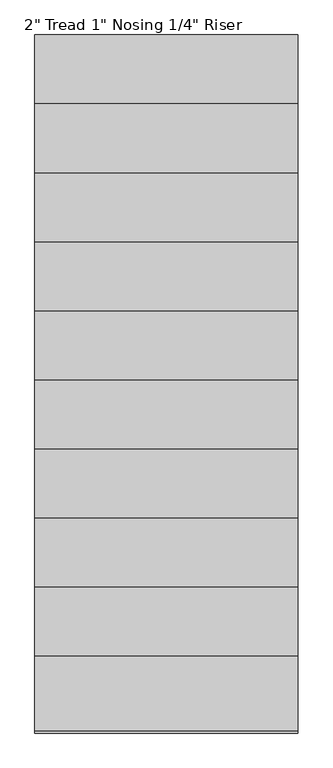
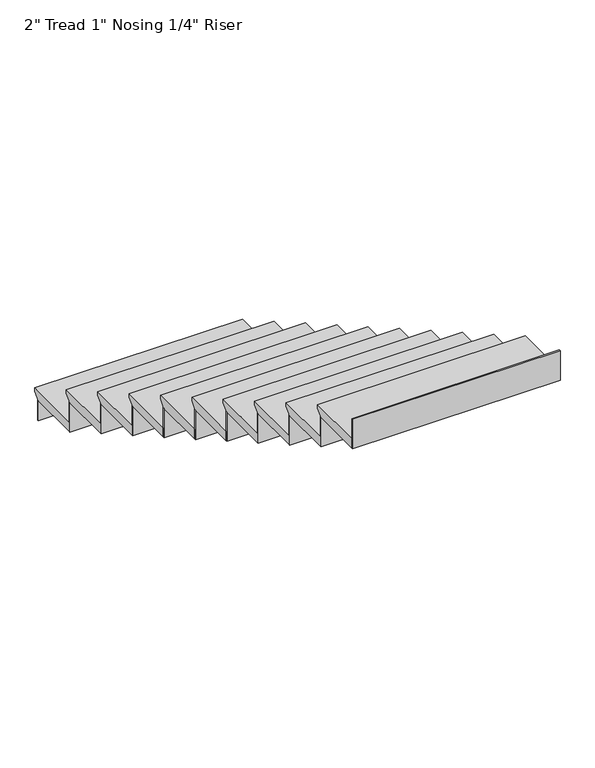
"""IFC4 building model written with IfcOpenShell, lengths in millimetres: stair flight geometry."""

from ifc_helpers import new_model, si_unit, origin, place, context, project, spatial, faceted_brep, source, transform, mapped, element, save


def stair_flight_b7621f50(model_context):
    return source(origin(), model_context, "Body", "Brep", [
        faceted_brep([(-6889.1581554, 6889.086641, 140.2772727), (-6889.1581554, 6889.086641, 159.3272727), (-5822.3581554, 6889.086641, 159.3272727), (-5822.3581554, 6889.086641, 140.2772727), (-6889.1581554, 6863.686641, 114.8772727), (-5822.3581554, 6863.686641, 114.8772727), (-6889.1581554, 6584.286641, 159.3272727), (-5822.3581554, 6584.286641, 159.3272727), (-5822.3581554, 6863.686641, 108.5272727), (-5822.3581554, 6584.286641, 108.5272727), (-6889.1581554, 6584.286641, 108.5272727), (-6889.1581554, 6863.686641, 108.5272727)], [[[0, 1, 2, 3]], [[4, 0, 3, 5]], [[2, 1, 6, 7]], [[8, 9, 10, 11]], [[2, 7, 9, 8, 5, 3]], [[8, 11, 4, 5]], [[6, 1, 0, 4, 11, 10]], [[7, 6, 10, 9]]]),
        faceted_brep([(-6889.1581554, 6863.686641, 108.5272727), (-6889.1581554, 6863.686641, 0.0), (-6889.1581554, 6857.336641, 0.0), (-6889.1581554, 6857.336641, 108.5272727), (-5822.3581554, 6863.686641, 108.5272727), (-5822.3581554, 6857.336641, 108.5272727), (-5822.3581554, 6857.336641, 0.0), (-5822.3581554, 6863.686641, 0.0)], [[[0, 1, 2, 3]], [[4, 5, 6, 7]], [[1, 0, 4, 7]], [[2, 1, 7, 6]], [[3, 2, 6, 5]], [[0, 3, 5, 4]]]),
        faceted_brep([(-6889.1581554, 6584.286641, 267.8545455), (-6889.1581554, 6584.286641, 108.5272727), (-6889.1581554, 6577.936641, 108.5272727), (-6889.1581554, 6577.936641, 267.8545455), (-5822.3581554, 6584.286641, 267.8545455), (-5822.3581554, 6577.936641, 267.8545455), (-5822.3581554, 6577.936641, 108.5272727), (-5822.3581554, 6584.286641, 108.5272727)], [[[0, 1, 2, 3]], [[4, 5, 6, 7]], [[1, 0, 4, 7]], [[2, 1, 7, 6]], [[3, 2, 6, 5]], [[0, 3, 5, 4]]]),
        faceted_brep([(-5822.3581554, 6609.686641, 318.6545455), (-6889.1581554, 6609.686641, 318.6545455), (-6889.1581554, 6304.886641, 318.6545455), (-5822.3581554, 6304.886641, 318.6545455), (-5822.3581554, 6584.286641, 267.8545455), (-5822.3581554, 6304.886641, 267.8545455), (-6889.1581554, 6304.886641, 267.8545455), (-6889.1581554, 6584.286641, 267.8545455), (-5822.3581554, 6584.286641, 274.2045455), (-5822.3581554, 6609.686641, 299.6045455), (-6889.1581554, 6584.286641, 274.2045455), (-6889.1581554, 6609.686641, 299.6045455)], [[[0, 1, 2, 3]], [[4, 5, 6, 7]], [[0, 3, 5, 4, 8, 9]], [[4, 7, 10, 8]], [[2, 1, 11, 10, 7, 6]], [[3, 2, 6, 5]], [[11, 1, 0, 9]], [[10, 11, 9, 8]]]),
        faceted_brep([(-6889.1581554, 6304.886641, 427.1818182), (-6889.1581554, 6304.886641, 267.8545455), (-6889.1581554, 6298.536641, 267.8545455), (-6889.1581554, 6298.536641, 427.1818182), (-5822.3581554, 6304.886641, 427.1818182), (-5822.3581554, 6298.536641, 427.1818182), (-5822.3581554, 6298.536641, 267.8545455), (-5822.3581554, 6304.886641, 267.8545455)], [[[0, 1, 2, 3]], [[4, 5, 6, 7]], [[1, 0, 4, 7]], [[2, 1, 7, 6]], [[3, 2, 6, 5]], [[0, 3, 5, 4]]]),
        faceted_brep([(-5822.3581554, 6330.286641, 477.9818182), (-6889.1581554, 6330.286641, 477.9818182), (-6889.1581554, 6025.486641, 477.9818182), (-5822.3581554, 6025.486641, 477.9818182), (-5822.3581554, 6304.886641, 427.1818182), (-5822.3581554, 6025.486641, 427.1818182), (-6889.1581554, 6025.486641, 427.1818182), (-6889.1581554, 6304.886641, 427.1818182), (-5822.3581554, 6304.886641, 433.5318182), (-5822.3581554, 6330.286641, 458.9318182), (-6889.1581554, 6304.886641, 433.5318182), (-6889.1581554, 6330.286641, 458.9318182)], [[[0, 1, 2, 3]], [[4, 5, 6, 7]], [[0, 3, 5, 4, 8, 9]], [[4, 7, 10, 8]], [[2, 1, 11, 10, 7, 6]], [[3, 2, 6, 5]], [[11, 1, 0, 9]], [[10, 11, 9, 8]]]),
        faceted_brep([(-6889.1581554, 6025.486641, 586.5090909), (-6889.1581554, 6025.486641, 427.1818182), (-6889.1581554, 6019.136641, 427.1818182), (-6889.1581554, 6019.136641, 586.5090909), (-5822.3581554, 6025.486641, 586.5090909), (-5822.3581554, 6019.136641, 586.5090909), (-5822.3581554, 6019.136641, 427.1818182), (-5822.3581554, 6025.486641, 427.1818182)], [[[0, 1, 2, 3]], [[4, 5, 6, 7]], [[1, 0, 4, 7]], [[2, 1, 7, 6]], [[3, 2, 6, 5]], [[0, 3, 5, 4]]]),
        faceted_brep([(-5822.3581554, 6050.886641, 637.3090909), (-6889.1581554, 6050.886641, 637.3090909), (-6889.1581554, 5746.086641, 637.3090909), (-5822.3581554, 5746.086641, 637.3090909), (-5822.3581554, 6025.486641, 586.5090909), (-5822.3581554, 5746.086641, 586.5090909), (-6889.1581554, 5746.086641, 586.5090909), (-6889.1581554, 6025.486641, 586.5090909), (-5822.3581554, 6025.486641, 592.8590909), (-5822.3581554, 6050.886641, 618.2590909), (-6889.1581554, 6025.486641, 592.8590909), (-6889.1581554, 6050.886641, 618.2590909)], [[[0, 1, 2, 3]], [[4, 5, 6, 7]], [[0, 3, 5, 4, 8, 9]], [[4, 7, 10, 8]], [[2, 1, 11, 10, 7, 6]], [[3, 2, 6, 5]], [[11, 1, 0, 9]], [[10, 11, 9, 8]]]),
        faceted_brep([(-6889.1581554, 5746.086641, 745.8363636), (-6889.1581554, 5746.086641, 586.5090909), (-6889.1581554, 5739.736641, 586.5090909), (-6889.1581554, 5739.736641, 745.8363636), (-5822.3581554, 5746.086641, 745.8363636), (-5822.3581554, 5739.736641, 745.8363636), (-5822.3581554, 5739.736641, 586.5090909), (-5822.3581554, 5746.086641, 586.5090909)], [[[0, 1, 2, 3]], [[4, 5, 6, 7]], [[1, 0, 4, 7]], [[2, 1, 7, 6]], [[3, 2, 6, 5]], [[0, 3, 5, 4]]]),
        faceted_brep([(-5822.3581554, 5771.486641, 796.6363636), (-6889.1581554, 5771.486641, 796.6363636), (-6889.1581554, 5466.686641, 796.6363636), (-5822.3581554, 5466.686641, 796.6363636), (-5822.3581554, 5746.086641, 745.8363636), (-5822.3581554, 5466.686641, 745.8363636), (-6889.1581554, 5466.686641, 745.8363636), (-6889.1581554, 5746.086641, 745.8363636), (-5822.3581554, 5746.086641, 752.1863636), (-5822.3581554, 5771.486641, 777.5863636), (-6889.1581554, 5746.086641, 752.1863636), (-6889.1581554, 5771.486641, 777.5863636)], [[[0, 1, 2, 3]], [[4, 5, 6, 7]], [[0, 3, 5, 4, 8, 9]], [[4, 7, 10, 8]], [[2, 1, 11, 10, 7, 6]], [[3, 2, 6, 5]], [[11, 1, 0, 9]], [[10, 11, 9, 8]]]),
        faceted_brep([(-6889.1581554, 5466.686641, 905.1636364), (-6889.1581554, 5466.686641, 745.8363636), (-6889.1581554, 5460.336641, 745.8363636), (-6889.1581554, 5460.336641, 905.1636364), (-5822.3581554, 5466.686641, 905.1636364), (-5822.3581554, 5460.336641, 905.1636364), (-5822.3581554, 5460.336641, 745.8363636), (-5822.3581554, 5466.686641, 745.8363636)], [[[0, 1, 2, 3]], [[4, 5, 6, 7]], [[1, 0, 4, 7]], [[2, 1, 7, 6]], [[3, 2, 6, 5]], [[0, 3, 5, 4]]]),
        faceted_brep([(-5822.3581554, 5492.086641, 955.9636364), (-6889.1581554, 5492.086641, 955.9636364), (-6889.1581554, 5187.286641, 955.9636364), (-5822.3581554, 5187.286641, 955.9636364), (-5822.3581554, 5466.686641, 905.1636364), (-5822.3581554, 5187.286641, 905.1636364), (-6889.1581554, 5187.286641, 905.1636364), (-6889.1581554, 5466.686641, 905.1636364), (-5822.3581554, 5466.686641, 911.5136364), (-5822.3581554, 5492.086641, 936.9136364), (-6889.1581554, 5466.686641, 911.5136364), (-6889.1581554, 5492.086641, 936.9136364)], [[[0, 1, 2, 3]], [[4, 5, 6, 7]], [[0, 3, 5, 4, 8, 9]], [[4, 7, 10, 8]], [[2, 1, 11, 10, 7, 6]], [[3, 2, 6, 5]], [[11, 1, 0, 9]], [[10, 11, 9, 8]]]),
        faceted_brep([(-6889.1581554, 5187.286641, 1064.4909091), (-6889.1581554, 5187.286641, 905.1636364), (-6889.1581554, 5180.936641, 905.1636364), (-6889.1581554, 5180.936641, 1064.4909091), (-5822.3581554, 5187.286641, 1064.4909091), (-5822.3581554, 5180.936641, 1064.4909091), (-5822.3581554, 5180.936641, 905.1636364), (-5822.3581554, 5187.286641, 905.1636364)], [[[0, 1, 2, 3]], [[4, 5, 6, 7]], [[1, 0, 4, 7]], [[2, 1, 7, 6]], [[3, 2, 6, 5]], [[0, 3, 5, 4]]]),
        faceted_brep([(-5822.3581554, 5212.686641, 1115.2909091), (-6889.1581554, 5212.686641, 1115.2909091), (-6889.1581554, 4907.886641, 1115.2909091), (-5822.3581554, 4907.886641, 1115.2909091), (-5822.3581554, 5187.286641, 1064.4909091), (-5822.3581554, 4907.886641, 1064.4909091), (-6889.1581554, 4907.886641, 1064.4909091), (-6889.1581554, 5187.286641, 1064.4909091), (-5822.3581554, 5187.286641, 1070.8409091), (-5822.3581554, 5212.686641, 1096.2409091), (-6889.1581554, 5187.286641, 1070.8409091), (-6889.1581554, 5212.686641, 1096.2409091)], [[[0, 1, 2, 3]], [[4, 5, 6, 7]], [[0, 3, 5, 4, 8, 9]], [[4, 7, 10, 8]], [[2, 1, 11, 10, 7, 6]], [[3, 2, 6, 5]], [[11, 1, 0, 9]], [[10, 11, 9, 8]]]),
        faceted_brep([(-6889.1581554, 4907.886641, 1223.8181818), (-6889.1581554, 4907.886641, 1064.4909091), (-6889.1581554, 4901.536641, 1064.4909091), (-6889.1581554, 4901.536641, 1223.8181818), (-5822.3581554, 4907.886641, 1223.8181818), (-5822.3581554, 4901.536641, 1223.8181818), (-5822.3581554, 4901.536641, 1064.4909091), (-5822.3581554, 4907.886641, 1064.4909091)], [[[0, 1, 2, 3]], [[4, 5, 6, 7]], [[1, 0, 4, 7]], [[2, 1, 7, 6]], [[3, 2, 6, 5]], [[0, 3, 5, 4]]]),
        faceted_brep([(-5822.3581554, 4933.286641, 1274.6181818), (-6889.1581554, 4933.286641, 1274.6181818), (-6889.1581554, 4628.486641, 1274.6181818), (-5822.3581554, 4628.486641, 1274.6181818), (-5822.3581554, 4907.886641, 1223.8181818), (-5822.3581554, 4628.486641, 1223.8181818), (-6889.1581554, 4628.486641, 1223.8181818), (-6889.1581554, 4907.886641, 1223.8181818), (-5822.3581554, 4907.886641, 1230.1681818), (-5822.3581554, 4933.286641, 1255.5681818), (-6889.1581554, 4907.886641, 1230.1681818), (-6889.1581554, 4933.286641, 1255.5681818)], [[[0, 1, 2, 3]], [[4, 5, 6, 7]], [[0, 3, 5, 4, 8, 9]], [[4, 7, 10, 8]], [[2, 1, 11, 10, 7, 6]], [[3, 2, 6, 5]], [[11, 1, 0, 9]], [[10, 11, 9, 8]]]),
        faceted_brep([(-6889.1581554, 4628.486641, 1383.1454545), (-6889.1581554, 4628.486641, 1223.8181818), (-6889.1581554, 4622.136641, 1223.8181818), (-6889.1581554, 4622.136641, 1383.1454545), (-5822.3581554, 4628.486641, 1383.1454545), (-5822.3581554, 4622.136641, 1383.1454545), (-5822.3581554, 4622.136641, 1223.8181818), (-5822.3581554, 4628.486641, 1223.8181818)], [[[0, 1, 2, 3]], [[4, 5, 6, 7]], [[1, 0, 4, 7]], [[2, 1, 7, 6]], [[3, 2, 6, 5]], [[0, 3, 5, 4]]]),
        faceted_brep([(-5822.3581554, 4653.886641, 1433.9454545), (-6889.1581554, 4653.886641, 1433.9454545), (-6889.1581554, 4349.086641, 1433.9454545), (-5822.3581554, 4349.086641, 1433.9454545), (-5822.3581554, 4628.486641, 1383.1454545), (-5822.3581554, 4349.086641, 1383.1454545), (-6889.1581554, 4349.086641, 1383.1454545), (-6889.1581554, 4628.486641, 1383.1454545), (-5822.3581554, 4628.486641, 1389.4954545), (-5822.3581554, 4653.886641, 1414.8954545), (-6889.1581554, 4628.486641, 1389.4954545), (-6889.1581554, 4653.886641, 1414.8954545)], [[[0, 1, 2, 3]], [[4, 5, 6, 7]], [[0, 3, 5, 4, 8, 9]], [[4, 7, 10, 8]], [[2, 1, 11, 10, 7, 6]], [[3, 2, 6, 5]], [[11, 1, 0, 9]], [[10, 11, 9, 8]]]),
        faceted_brep([(-6889.1581554, 4069.686641, 1701.8), (-6889.1581554, 4069.686641, 1542.4727273), (-6889.1581554, 4063.336641, 1542.4727273), (-6889.1581554, 4063.336641, 1701.8), (-5822.3581554, 4069.686641, 1701.8), (-5822.3581554, 4063.336641, 1701.8), (-5822.3581554, 4063.336641, 1542.4727273), (-5822.3581554, 4069.686641, 1542.4727273)], [[[0, 1, 2, 3]], [[4, 5, 6, 7]], [[1, 0, 4, 7]], [[2, 1, 7, 6]], [[3, 2, 6, 5]], [[0, 3, 5, 4]]]),
        faceted_brep([(-6889.1581554, 4349.086641, 1542.4727273), (-6889.1581554, 4349.086641, 1383.1454545), (-6889.1581554, 4342.736641, 1383.1454545), (-6889.1581554, 4342.736641, 1542.4727273), (-5822.3581554, 4349.086641, 1542.4727273), (-5822.3581554, 4342.736641, 1542.4727273), (-5822.3581554, 4342.736641, 1383.1454545), (-5822.3581554, 4349.086641, 1383.1454545)], [[[0, 1, 2, 3]], [[4, 5, 6, 7]], [[1, 0, 4, 7]], [[2, 1, 7, 6]], [[3, 2, 6, 5]], [[0, 3, 5, 4]]]),
        faceted_brep([(-5822.3581554, 4069.686641, 1593.2727273), (-5822.3581554, 4095.086641, 1593.2727273), (-5822.3581554, 4374.486641, 1593.2727273), (-6889.1581554, 4374.486641, 1593.2727273), (-6889.1581554, 4069.686641, 1593.2727273), (-5822.3581554, 4095.086641, 1542.4727273), (-5822.3581554, 4069.686641, 1542.4727273), (-6889.1581554, 4069.686641, 1542.4727273), (-6889.1581554, 4349.086641, 1542.4727273), (-5822.3581554, 4349.086641, 1542.4727273), (-5822.3581554, 4349.086641, 1548.8227273), (-5822.3581554, 4374.486641, 1574.2227273), (-6889.1581554, 4349.086641, 1548.8227273), (-6889.1581554, 4374.486641, 1574.2227273)], [[[0, 1, 2, 3, 4]], [[5, 6, 7, 8, 9]], [[1, 0, 6, 5]], [[2, 1, 5, 9, 10, 11]], [[9, 8, 12, 10]], [[4, 3, 13, 12, 8, 7]], [[0, 4, 7, 6]], [[13, 3, 2, 11]], [[12, 13, 11, 10]]]),
    ])


if __name__ == "__main__":
    model = new_model("IFC4")
    model_context = context("Model", 3, world=origin())
    ifc_project = project(units=[si_unit("LENGTHUNIT", "METRE", prefix="MILLI")], contexts=[model_context])
    site = spatial("IfcSite", under=ifc_project)
    building = spatial("IfcBuilding", under=site)
    placement = place(None, origin())
    stair_flight_shape = stair_flight_b7621f50(model_context)
    element("IfcStairFlight", 1, ObjectType="2\" Tread 1\" Nosing 1/4\" Riser", at=placement, inside=building, context=model_context, shape_type="MappedRepresentation", body=[
        mapped(stair_flight_shape, transform((0.0, 0.0, 0.0), x_axis=(1.0, 0.0, 0.0), y_axis=(0.0, 1.0, 0.0), z_axis=(0.0, 0.0, 1.0))),
    ])
    save(model, "model.ifc")
